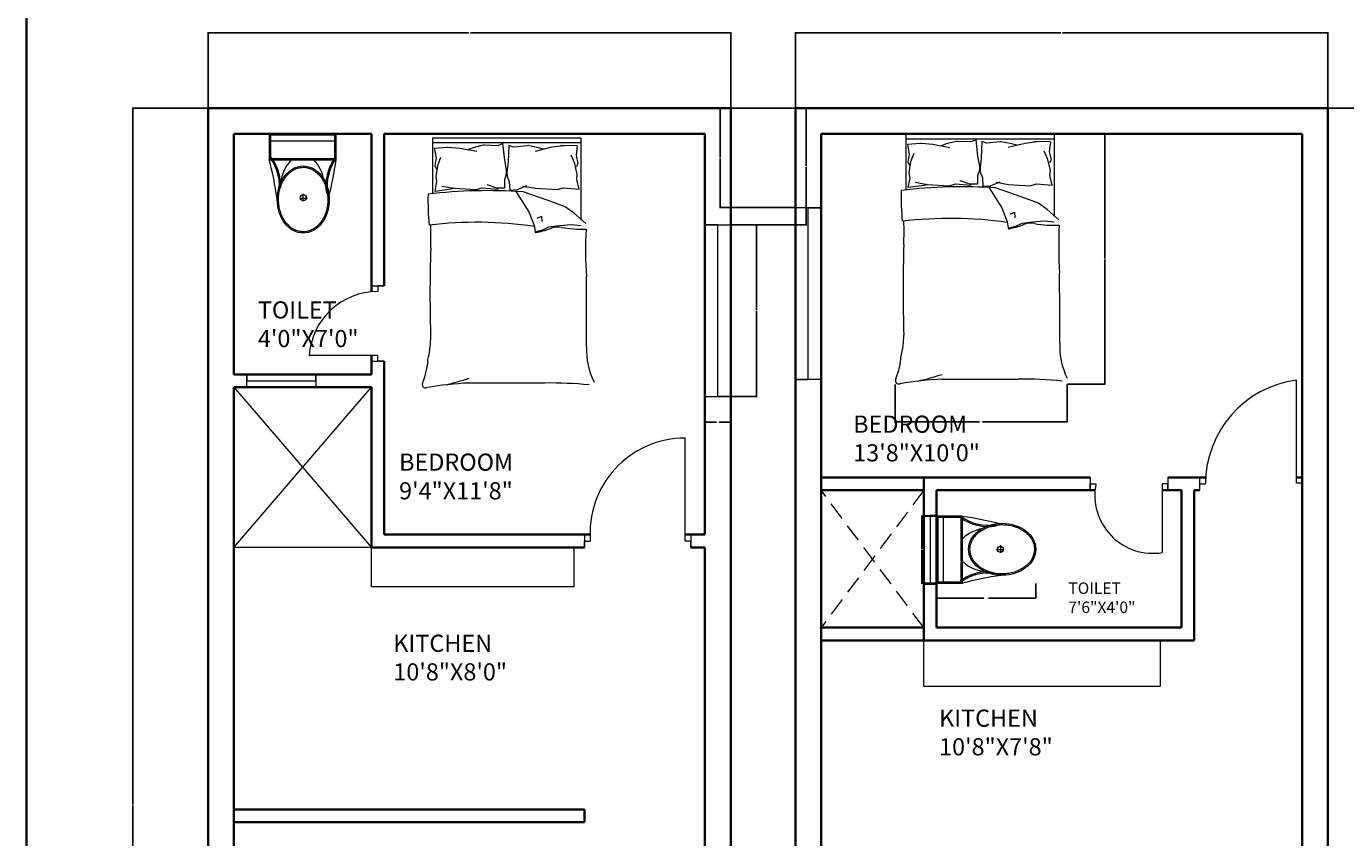
# Model space of a CAD drawing. Units: inches. Extents: x 2169 to 3181, y 1824 to 2912.
# Tile 2 of 5: x 2169 to 2630, y 2163 to 2446. Entities that reach past the tile are written whole.
import ezdxf

# ---------------------------------------------------------------- set-up
doc = ezdxf.new("R2010")
doc.units = ezdxf.units.IN
doc.linetypes.add('DASHED2', pattern=[9.525, 6.35, -3.175])
for name, color, linetype, lineweight in [('A-ANNO-DIMS', 2, 'Continuous', 18), ('A-ANNO-TTLB', 7, 'Continuous', 35), ('A-AREA-IDEN', 7, 'Continuous', 18), ('A-DOOR', 3, 'Continuous', 18), ('A-FLOR-CASE', 8, 'Continuous', 18), ('A-FLOR-FIXT', 9, 'Continuous', 18), ('A-FLOR-OPEN', 7, 'Continuous', 18), ('A-FLOR-OPEN-OVHD', 253, 'DASHED2', 13), ('A-FURN', 8, 'Continuous', 18), ('A-GLAZ', 4, 'Continuous', 18), ('A-WALL', 7, 'Continuous', 35)]:
    doc.layers.add(name, color=color, linetype=linetype, lineweight=lineweight)
doc.styles.get("Standard").update_dxf_attribs({"font": 'arial.ttf'})
doc.dimstyles.get("Standard").update_dxf_attribs({"dimtxt": 0.18, "dimasz": 0.18, "dimexe": 0.18, "dimexo": 0.0625, "dimgap": 0.09, "dimtad": 0, "dimtih": 1, "dimtoh": 1, "dimdec": 4, "dimzin": 0, "dimdsep": 46, "dimtxsty": 'Standard', "dimcen": 0.09, "dimadec": 0, "dimazin": 0, "dimtfac": 1, "dimtdec": 4, "dimtofl": 0, "dimtmove": 0, "dimatfit": 3, "dimfxl": 1, "dimtolj": 1, "dimtzin": 0, "dimarcsym": 0})

# ---------------------------------------------------------------- blocks, each defined once
blk = doc.blocks.new('A$C31115884')
for p, q in [((258, 466), (258, 523)), ((283, 498), (223, 498)), ((0, 200), (0, 0)), ((520, 200), (0, 200)), ((10, 190), (10, 10)), ((510, 190), (10, 190)), ((510, 10), (510, 190)), ((520, 0), (520, 200)), ((510, 54), (0, 54)), ((10, 10), (510, 10)), ((0, 0), (520, 0))]:
    blk.add_line(p, q)
blk.add_circle((256, 496), 23.6)
for centre, radius, start, end in [((2778, -205), 2807, 165.4549, 171.7133), ((-295, 403), 365, 324.2091, 9.3499), ((-295, 403), 375, 324.2091, 9.3499), ((139, 406), 293, 315.8436, 2.6563), ((806, 403), 365, 170.6501, 215.7909), ((3237, 905), 2807, 188.2867, 194.5451), ((384, 406), 293, 190.2774, 224.1564), ((806, 403), 375, 179.2036, 215.7909)]:
    blk.add_arc(centre, radius, start, end)
blk.add_ellipse((256, 510), major_axis=(0, -261), ratio=0.772727)
blk.add_open_spline([(256, 259), (263, 259), (270, 260), (288, 262), (299, 265), (320, 273), (330, 278), (350, 291), (360, 299), (378, 316), (386, 326), (402, 347), (409, 358), (421, 383), (427, 395), (436, 422), (440, 436), (445, 465), (447, 480), (448, 509), (448, 524), (445, 553), (443, 568), (436, 596), (432, 610), (422, 636), (416, 649), (402, 672), (395, 683), (379, 703), (370, 712), (351, 728), (341, 735), (321, 746), (310, 751), (289, 757), (278, 759), (256, 761), (245, 761), (223, 757), (212, 754), (191, 746), (181, 741), (161, 728), (151, 720), (133, 703), (125, 693), (110, 672), (103, 660), (90, 636), (85, 623), (76, 596), (72, 582), (67, 553), (66, 538), (64, 509), (65, 494), (68, 465), (70, 450), (77, 422), (81, 408), (91, 382), (97, 370), (111, 346), (118, 335), (135, 316), (144, 307), (162, 291), (172, 284), (193, 273), (203, 269), (225, 262), (236, 260), (250, 259), (253, 259), (256, 259)], degree=3, knots=[0, 0, 0, 0, 0.110105, 0.110105, 0.285049, 0.285049, 0.459994, 0.459994, 0.634938, 0.634938, 0.809882, 0.809882, 0.984827, 0.984827, 1.159771, 1.159771, 1.334715, 1.334715, 1.50966, 1.50966, 1.684604, 1.684604, 1.859549, 1.859549, 2.034493, 2.034493, 2.209437, 2.209437, 2.384382, 2.384382, 2.559326, 2.559326, 2.73427, 2.73427, 2.909215, 2.909215, 3.084159, 3.084159, 3.259103, 3.259103, 3.434048, 3.434048, 3.608992, 3.608992, 3.783936, 3.783936, 3.958881, 3.958881, 4.133825, 4.133825, 4.30877, 4.30877, 4.483714, 4.483714, 4.658658, 4.658658, 4.833603, 4.833603, 5.008547, 5.008547, 5.183491, 5.183491, 5.358436, 5.358436, 5.53338, 5.53338, 5.708324, 5.708324, 5.883269, 5.883269, 6.058213, 6.058213, 6.233158, 6.233158, 6.283185, 6.283185, 6.283185, 6.283185])
blk = doc.blocks.new('DOOR-BED-G-36IN')
for p, q in [((0, 0), (0, 36)), ((-35.15, 2.25), (-35.15, -2.25)), ((2, 2.25), (2, -2.25)), ((-35.15, -2.25), (-35.15, 0)), ((-35.15, 0), (-33.15, 0)), ((2, 0), (0, 0)), ((2, -2.25), (2, 0))]:
    blk.add_line(p, q)
blk.add_arc((0, 2.74), 33.26, 90, 184.7229)
blk = doc.blocks.new('DOOR-BATH-G-24IN')
for p, q in [((-2.25, 24.37), (2.25, 24.37)), ((2.25, 24.37), (0, 24.37)), ((0, 24.37), (0, 22.37)), ((0, 0), (-24, 0)), ((0, -2), (0, 0)), ((-2.25, -2), (-2.25, -2)), ((-2.25, -2), (2.25, -2)), ((2.25, -2), (0, -2))]:
    blk.add_line(p, q)
blk.add_arc((0, -1.69), 24.06, 90, 175.9745)
blk = doc.blocks.new('DOOR-BATH-U-24IN')
for p, q in [((-25.15, 2.25), (-25.15, -2.25)), ((2, 2.25), (2, -2.25)), ((-25.15, -2.25), (-25.15, 0)), ((-25.15, 0), (-23.15, 0)), ((2, 0), (0, 0)), ((0, 0), (0, -24)), ((2, -2.25), (2, 0))]:
    blk.add_line(p, q)
blk.add_arc((-3.27, -3.99), 20.28, 168.6528, 279.2746)
blk = doc.blocks.new('DOOR-BED-U-36IN')
for p, q in [((0, 0), (0, 36)), ((-33.79, -2.49), (-33.79, 2.01)), ((-33.79, 2.01), (-33.79, 2.01)), ((2, 0), (0, 0)), ((-33.79, -0.24), (-31.79, -0.24)), ((-33.79, -2.49), (-33.79, -2.49))]:
    blk.add_line(p, q)
blk.add_arc((4.76, -0.24), 36.56, 97.4851, 180)
blk = doc.blocks.new('WIN-60IN')
for p, q in [((4.5, 60), (0, 60)), ((0, 60), (9, 60)), ((4.5, 0), (4.5, 60)), ((0, 0), (9, 0)), ((9, 0), (4.5, 0)), ((9, 0), (9, 0))]:
    blk.add_line(p, q)
blk = doc.blocks.new('VENT-24IN-G')
for p, q in [((0, 0), (0, 4.5)), ((0, 4.5), (0, 2.25)), ((0, 2.25), (24, 2.25)), ((24, 2.25), (24, 4.5)), ((24, 4.5), (24, 0))]:
    blk.add_line(p, q)
blk = doc.blocks.new('VENT-24IN-U')
for p, q in [((0, 24), (0, 24)), ((0, 24), (4.5, 24)), ((4.5, 24), (2.25, 24)), ((2.25, 24), (2.25, 0)), ((2.25, 0), (0, 0)), ((0, 0), (4.5, 0))]:
    blk.add_line(p, q)
blk = doc.blocks.new('BED-DOUBLE')
for p, q in [((3.76, 67.77), (3.76, 87.35)), ((3.76, 87.35), (55.42, 87.35)), ((3.76, 85.69), (55.42, 85.69)), ((4.21, 83.74), (8.84, 84.1)), ((4.21, 83.77), (4.83, 80.33)), ((8.84, 84.1), (8.96, 84.08)), ((8.96, 84.08), (13.09, 83.77)), ((13.09, 83.77), (19.03, 82.67)), ((16.06, 83.3), (18.25, 84.08)), ((18.25, 84.08), (21.37, 84.86)), ((21.37, 84.86), (21.72, 84.86)), ((21.72, 84.86), (26.52, 84.7)), ((26.52, 84.7), (28.09, 85.33)), ((28.09, 85.33), (28.71, 79.55)), ((30.24, 84.66), (29.98, 78.85)), ((31.84, 84.13), (30.24, 84.66)), ((36.63, 84.59), (31.84, 84.13)), ((36.98, 84.61), (36.63, 84.59)), ((40.14, 84.02), (36.98, 84.61)), ((45.31, 84.03), (39.45, 82.57)), ((42.38, 83.38), (40.14, 84.02)), ((49.42, 84.6), (45.31, 84.03)), ((54.17, 84.59), (48.33, 84.69)), ((48.33, 84.69), (49.42, 84.6)), ((54.17, 84.59), (53.76, 81.12)), ((55.42, 87.35), (55.42, 58.59)), ((4.83, 80.33), (4.37, 77.51)), ((5.46, 77.67), (6.55, 80.64)), ((28.71, 79.55), (29.34, 76.11)), ((29.98, 78.85), (29.57, 75.38)), ((53.3, 78.42), (52.03, 81.32)), ((54.17, 74.56), (53.3, 78.42)), ((53.76, 81.12), (54.41, 78.34)), ((54.41, 78.34), (53.85, 77.21)), ((4.37, 77.51), (4.99, 76.42)), ((4.83, 73.76), (5.46, 77.67)), ((5.15, 72.04), (4.83, 73.76)), ((29.34, 74.7), (28.71, 72.67)), ((29.34, 76.11), (29.34, 74.7)), ((29.57, 75.38), (29.66, 73.97)), ((29.66, 73.97), (30.41, 71.98)), ((53.97, 72.83), (54.17, 74.56)), ((4.52, 68.6), (5.15, 72.04)), ((10.03, 69.39), (4.52, 68.6)), ((6.9, 70.46), (11.26, 69.74)), ((11.26, 69.74), (10.03, 69.39)), ((11.26, 69.74), (18.83, 69.27)), ((18.83, 69.27), (20.95, 69.87)), ((20.95, 69.87), (26.5, 69.44)), ((26.06, 69.77), (22.66, 70.95)), ((28.71, 69.77), (26.06, 69.77)), ((28.71, 72.67), (28.71, 69.77)), ((30.41, 71.98), (30.59, 69.09)), ((30.59, 69.09), (33.24, 69.26)), ((33.24, 69.26), (36.56, 70.64)), ((35.2, 70.46), (39.56, 69.74)), ((39.56, 69.74), (47.14, 69.27)), ((47.14, 69.27), (49.26, 69.87)), ((49.26, 69.87), (54.81, 69.44)), ((54.81, 69.44), (53.97, 72.83)), ((32.71, 68.56), (37.24, 61.54)), ((43.94, 65.39), (34.92, 68.56)), ((49.96, 63.21), (43.94, 65.39)), ((37.24, 61.54), (39.08, 56.69)), ((40.12, 59.32), (41.78, 59.99)), ((41.87, 58.1), (41.78, 59.99, 4.18)), ((53.15, 60.87), (49.96, 63.21)), ((57.15, 57.36), (53.15, 60.87)), ((39.08, 56.69), (39.42, 54.51)), ((42.1, 55.18), (44.27, 56.19)), ((44.27, 56.19), (47.96, 56.69)), ((47.96, 56.69), (52.14, 57.02)), ((52.14, 57.02), (55.49, 56.69)), ((39.42, 54.51), (42.1, 55.18)), ((16.28, 1.69), (42.89, 1.69))]:
    blk.add_line(p, q)
for centre, radius, start, end in [((92.06, 65.63), 90.06, 178.7218, 185.604), ((23.09, -109.45), 178.34, 86.0865, 96.7821), ((19.19, -81.63), 139.47, 81.7845, 96.9006), ((-180.86, 53.65), 183.89, 358.4762, 1.0082), ((33.68, 85.75), 32.06, 280.6617, 289.8806), ((47.29, 49.44), 6.73, 78.6608, 113.7384), ((55.49, 94.55), 39.11, 259.8763, 272.5657), ((197.03, 48.09), 139.99, 176.9791, 183.8365), ((39.6, 54.45), 0.199, 160.2464, 271.1377), ((524.1, 32.64), 521.39, 178.2277, 181.7185), ((-4874.07, 14.03), 4931.49, 0.00217, 0.28689), ((-29.08, 17.61), 32.04, 346.0648, 358.9113), ((82.33, 13.12), 24.93, 177.4714, 206.4681), ((-23.41, 11.38), 25.47, 337.9751, 356.652), ((1.18, 1.17), 1.18, 146.1736, 293.4781), ((23.16, -129.76), 131.62, 92.9958, 99.4091), ((-18.62, 112.98), 115.08, 283.3832, 287.7053), ((44.49, -142.13), 143.82, 84.4998, 90.6351)]:
    blk.add_arc(centre, radius, start, end)
blk = doc.blocks.new('*D19')
at = {"layer": 'A-ANNO-DIMS', "color": 0, "lineweight": -2, "transparency": 16777216}
for p, q in [((2414.84, 2376.69), (2423.95, 2376.69)), ((2423.77, 2376.51), (2423.77, 2346.87)), ((2423.77, 2316.87), (2423.77, 2346.51)), ((2414.84, 2316.69), (2423.95, 2316.69))]:
    blk.add_line(p, q, dxfattribs=at)
at = {"layer": 'A-ANNO-DIMS', "color": 0, "transparency": 16777216}
for points in [[(2423.74, 2376.51), (2423.8, 2376.51), (2423.77, 2376.69)], [(2423.74, 2316.87), (2423.8, 2316.87), (2423.77, 2316.69)]]:
    blk.add_solid(points, dxfattribs=at)
at = {"layer": 'Defpoints', "color": 0, "transparency": 16777216}
for p in [(2414.77, 2376.69), (2423.77, 2376.69), (2414.77, 2316.69)]:
    blk.add_point(p, dxfattribs=at)
at = {"layer": 'A-ANNO-DIMS', "color": 0, "transparency": 16777216, "insert": (2423.77, 2346.69), "char_height": 0.18, "attachment_point": 5}
blk.add_mtext('\\A1;WINDOW 60 TYP.', dxfattribs=at)
blk = doc.blocks.new('*D20')
at = {"layer": 'A-ANNO-DIMS', "color": 0, "lineweight": -2, "transparency": 16777216}
for p, q in [((2405.77, 2316.63), (2405.77, 2307.51)), ((2414.77, 2316.63), (2414.77, 2307.51)), ((2405.95, 2307.69), (2409.82, 2307.69)), ((2414.59, 2307.69), (2410.73, 2307.69))]:
    blk.add_line(p, q, dxfattribs=at)
at = {"layer": 'A-ANNO-DIMS', "color": 0, "transparency": 16777216}
for points in [[(2405.95, 2307.72), (2405.95, 2307.66), (2405.77, 2307.69)], [(2414.59, 2307.72), (2414.59, 2307.66), (2414.77, 2307.69)]]:
    blk.add_solid(points, dxfattribs=at)
at = {"layer": 'Defpoints', "color": 0, "transparency": 16777216}
for p in [(2405.77, 2316.69), (2414.77, 2316.69), (2414.77, 2307.69)]:
    blk.add_point(p, dxfattribs=at)
at = {"layer": 'A-ANNO-DIMS', "color": 0, "transparency": 16777216, "insert": (2410.27, 2307.69), "char_height": 0.18, "attachment_point": 5}
blk.add_mtext('\\A1;9 TYP.', dxfattribs=at)
blk = doc.blocks.new('*D43')
at = {"layer": 'A-ANNO-DIMS', "color": 0, "lineweight": -2, "transparency": 16777216}
for p, q in [((2486.67, 2251.35), (2486.67, 2246.04)), ((2521.31, 2251.35), (2521.31, 2246.04)), ((2486.85, 2246.22), (2503.21, 2246.22)), ((2521.13, 2246.22), (2504.77, 2246.22))]:
    blk.add_line(p, q, dxfattribs=at)
at = {"layer": 'A-ANNO-DIMS', "color": 0, "transparency": 16777216}
for points in [[(2486.85, 2246.25), (2486.85, 2246.19), (2486.67, 2246.22)], [(2521.13, 2246.25), (2521.13, 2246.19), (2521.31, 2246.22)]]:
    blk.add_solid(points, dxfattribs=at)
at = {"layer": 'Defpoints', "color": 0, "transparency": 16777216}
for p in [(2486.67, 2251.42), (2521.31, 2251.42), (2521.31, 2246.22)]:
    blk.add_point(p, dxfattribs=at)
at = {"layer": 'A-ANNO-DIMS', "color": 0, "transparency": 16777216, "insert": (2503.99, 2246.22), "char_height": 0.18, "attachment_point": 5}
blk.add_mtext('\\A1;WC 35 TYP.', dxfattribs=at)
blk = doc.blocks.new('*D44')
at = {"layer": 'A-ANNO-DIMS', "color": 0, "lineweight": -2, "transparency": 16777216}
for p, q in [((2486.61, 2274.79), (2481.29, 2274.79)), ((2481.47, 2274.61), (2481.47, 2263.29)), ((2481.47, 2251.6), (2481.47, 2262.92)), ((2486.61, 2251.42), (2481.29, 2251.42))]:
    blk.add_line(p, q, dxfattribs=at)
at = {"layer": 'A-ANNO-DIMS', "color": 0, "transparency": 16777216}
for points in [[(2481.44, 2274.61), (2481.5, 2274.61), (2481.47, 2274.79)], [(2481.44, 2251.6), (2481.5, 2251.6), (2481.47, 2251.42)]]:
    blk.add_solid(points, dxfattribs=at)
at = {"layer": 'Defpoints', "color": 0, "transparency": 16777216}
for p in [(2486.67, 2274.79), (2481.47, 2251.42), (2486.67, 2251.42)]:
    blk.add_point(p, dxfattribs=at)
at = {"layer": 'A-ANNO-DIMS', "color": 0, "transparency": 16777216, "insert": (2481.47, 2263.11), "char_height": 0.18, "attachment_point": 5}
blk.add_mtext('\\A1;23 TYP.', dxfattribs=at)
blk = doc.blocks.new('*D45')
at = {"layer": 'A-ANNO-DIMS', "color": 0, "lineweight": -2, "transparency": 16777216}
for p, q in [((2532.34, 2408.39), (2545.57, 2408.39)), ((2545.39, 2408.21), (2545.39, 2364.84)), ((2545.39, 2321.11), (2545.39, 2364.48)), ((2532.34, 2320.93), (2545.57, 2320.93))]:
    blk.add_line(p, q, dxfattribs=at)
at = {"layer": 'A-ANNO-DIMS', "color": 0, "transparency": 16777216}
for points in [[(2545.36, 2408.21), (2545.42, 2408.21), (2545.39, 2408.39)], [(2545.36, 2321.11), (2545.42, 2321.11), (2545.39, 2320.93)]]:
    blk.add_solid(points, dxfattribs=at)
at = {"layer": 'Defpoints', "color": 0, "transparency": 16777216}
for p in [(2532.27, 2408.39), (2545.39, 2408.39), (2532.27, 2320.93)]:
    blk.add_point(p, dxfattribs=at)
at = {"layer": 'A-ANNO-DIMS', "color": 0, "transparency": 16777216, "insert": (2545.39, 2364.66), "char_height": 0.18, "attachment_point": 5}
blk.add_mtext('\\A1;BED 87 TYP.', dxfattribs=at)
blk = doc.blocks.new('*D46')
at = {"layer": 'A-ANNO-DIMS', "color": 0, "lineweight": -2, "transparency": 16777216}
for p, q in [((2472.17, 2320.86), (2472.17, 2307.63)), ((2532.27, 2320.86), (2532.27, 2307.63)), ((2472.35, 2307.81), (2501.69, 2307.81)), ((2532.09, 2307.81), (2502.75, 2307.81))]:
    blk.add_line(p, q, dxfattribs=at)
at = {"layer": 'A-ANNO-DIMS', "color": 0, "transparency": 16777216}
for points in [[(2472.35, 2307.84), (2472.35, 2307.78), (2472.17, 2307.81)], [(2532.09, 2307.84), (2532.09, 2307.78), (2532.27, 2307.81)]]:
    blk.add_solid(points, dxfattribs=at)
at = {"layer": 'Defpoints', "color": 0, "transparency": 16777216}
for p in [(2472.17, 2320.93), (2532.27, 2320.93), (2532.27, 2307.81)]:
    blk.add_point(p, dxfattribs=at)
at = {"layer": 'A-ANNO-DIMS', "color": 0, "transparency": 16777216, "insert": (2502.22, 2307.81), "char_height": 0.18, "attachment_point": 5}
blk.add_mtext('\\A1;60 TYP.', dxfattribs=at)
blk = doc.blocks.new('*D53')
at = {"layer": 'A-ANNO-DIMS', "color": 0, "lineweight": -2, "transparency": 16777216}
for p, q in [((2232.27, 2417.45), (2232.27, 2443.92)), ((2232.45, 2443.74), (2323.14, 2443.74)), ((2414.59, 2443.74), (2323.91, 2443.74)), ((2414.77, 2417.45), (2414.77, 2443.92))]:
    blk.add_line(p, q, dxfattribs=at)
at = {"layer": 'A-ANNO-DIMS', "color": 0, "transparency": 16777216}
for points in [[(2232.45, 2443.77), (2232.45, 2443.71), (2232.27, 2443.74)], [(2414.59, 2443.77), (2414.59, 2443.71), (2414.77, 2443.74)]]:
    blk.add_solid(points, dxfattribs=at)
at = {"layer": 'Defpoints', "color": 0, "transparency": 16777216}
for p in [(2414.77, 2443.74), (2232.27, 2417.39), (2414.77, 2417.39)]:
    blk.add_point(p, dxfattribs=at)
at = {"layer": 'A-ANNO-DIMS', "color": 0, "transparency": 16777216, "insert": (2323.52, 2443.74), "char_height": 0.18, "attachment_point": 5}
blk.add_mtext('\\A1;182.5', dxfattribs=at)
blk = doc.blocks.new('*D54')
at = {"layer": 'A-ANNO-DIMS', "color": 0, "lineweight": -2, "transparency": 16777216}
for p, q in [((2232.21, 2417.39), (2205.74, 2417.39)), ((2205.92, 2417.21), (2205.92, 2174.07)), ((2205.92, 1930.57), (2205.92, 2173.71)), ((2232.21, 1930.39), (2205.74, 1930.39))]:
    blk.add_line(p, q, dxfattribs=at)
at = {"layer": 'A-ANNO-DIMS', "color": 0, "transparency": 16777216}
for points in [[(2205.89, 2417.21), (2205.95, 2417.21), (2205.92, 2417.39)], [(2205.89, 1930.57), (2205.95, 1930.57), (2205.92, 1930.39)]]:
    blk.add_solid(points, dxfattribs=at)
at = {"layer": 'Defpoints', "color": 0, "transparency": 16777216}
for p in [(2205.92, 2417.39), (2232.27, 2417.39), (2232.27, 1930.39)]:
    blk.add_point(p, dxfattribs=at)
at = {"layer": 'A-ANNO-DIMS', "color": 0, "transparency": 16777216, "insert": (2205.92, 2173.89), "char_height": 0.18, "attachment_point": 5}
blk.add_mtext('\\A1;487', dxfattribs=at)
blk = doc.blocks.new('*D55')
at = {"layer": 'A-ANNO-DIMS', "color": 0, "lineweight": -2, "transparency": 16777216}
for p, q in [((2437.37, 2417.45), (2437.37, 2443.92)), ((2437.55, 2443.74), (2530.09, 2443.74)), ((2623.19, 2443.74), (2530.65, 2443.74)), ((2623.37, 2417.45), (2623.37, 2443.92))]:
    blk.add_line(p, q, dxfattribs=at)
at = {"layer": 'A-ANNO-DIMS', "color": 0, "transparency": 16777216}
for points in [[(2437.55, 2443.77), (2437.55, 2443.71), (2437.37, 2443.74)], [(2623.19, 2443.77), (2623.19, 2443.71), (2623.37, 2443.74)]]:
    blk.add_solid(points, dxfattribs=at)
at = {"layer": 'Defpoints', "color": 0, "transparency": 16777216}
for p in [(2623.37, 2443.74), (2437.37, 2417.39), (2623.37, 2417.39)]:
    blk.add_point(p, dxfattribs=at)
at = {"layer": 'A-ANNO-DIMS', "color": 0, "transparency": 16777216, "insert": (2530.37, 2443.74), "char_height": 0.18, "attachment_point": 5}
blk.add_mtext('\\A1;186', dxfattribs=at)
blk = doc.blocks.new('*D56')
at = {"layer": 'A-ANNO-DIMS', "color": 0, "lineweight": -2, "transparency": 16777216}
for p, q in [((2623.43, 2417.39), (2649.9, 2417.39)), ((2649.72, 2417.21), (2649.72, 2174.07)), ((2649.72, 1930.57), (2649.72, 2173.71)), ((2623.43, 1930.39), (2649.9, 1930.39))]:
    blk.add_line(p, q, dxfattribs=at)
at = {"layer": 'A-ANNO-DIMS', "color": 0, "transparency": 16777216}
for points in [[(2649.69, 2417.21), (2649.75, 2417.21), (2649.72, 2417.39)], [(2649.69, 1930.57), (2649.75, 1930.57), (2649.72, 1930.39)]]:
    blk.add_solid(points, dxfattribs=at)
at = {"layer": 'Defpoints', "color": 0, "transparency": 16777216}
for p in [(2623.37, 2417.39), (2649.72, 2417.39), (2623.37, 1930.39)]:
    blk.add_point(p, dxfattribs=at)
at = {"layer": 'A-ANNO-DIMS', "color": 0, "transparency": 16777216, "insert": (2649.72, 2173.89), "char_height": 0.18, "attachment_point": 5}
blk.add_mtext('\\A1;487', dxfattribs=at)
blk = doc.blocks.new('*D57')
at = {"layer": 'A-ANNO-DIMS', "color": 0, "lineweight": -2, "transparency": 16777216}
for p, q in [((2414.84, 2417.39), (2441.3, 2417.39)), ((2441.12, 2417.21), (2441.12, 2397.22)), ((2441.12, 2376.87), (2441.12, 2396.86)), ((2414.84, 2376.69), (2441.3, 2376.69))]:
    blk.add_line(p, q, dxfattribs=at)
at = {"layer": 'A-ANNO-DIMS', "color": 0, "transparency": 16777216}
for points in [[(2441.09, 2417.21), (2441.15, 2417.21), (2441.12, 2417.39)], [(2441.09, 2376.87), (2441.15, 2376.87), (2441.12, 2376.69)]]:
    blk.add_solid(points, dxfattribs=at)
at = {"layer": 'Defpoints', "color": 0, "transparency": 16777216}
for p in [(2414.77, 2417.39), (2414.77, 2376.69), (2441.12, 2376.69)]:
    blk.add_point(p, dxfattribs=at)
at = {"layer": 'A-ANNO-DIMS', "color": 0, "transparency": 16777216, "insert": (2441.12, 2397.04), "char_height": 0.18, "attachment_point": 5}
blk.add_mtext('\\A1;40.7', dxfattribs=at)
blk = doc.blocks.new('*D58')
at = {"layer": 'A-ANNO-DIMS', "color": 0, "lineweight": -2, "transparency": 16777216}
for p, q in [((2437.31, 2417.39), (2410.84, 2417.39)), ((2411.02, 2417.21), (2411.02, 2400.2)), ((2411.02, 2382.82), (2411.02, 2399.83)), ((2437.31, 2382.64), (2410.84, 2382.64))]:
    blk.add_line(p, q, dxfattribs=at)
at = {"layer": 'A-ANNO-DIMS', "color": 0, "transparency": 16777216}
for points in [[(2410.99, 2417.21), (2411.05, 2417.21), (2411.02, 2417.39)], [(2410.99, 2382.82), (2411.05, 2382.82), (2411.02, 2382.64)]]:
    blk.add_solid(points, dxfattribs=at)
at = {"layer": 'Defpoints', "color": 0, "transparency": 16777216}
for p in [(2437.37, 2417.39), (2411.02, 2382.64), (2437.37, 2382.64)]:
    blk.add_point(p, dxfattribs=at)
at = {"layer": 'A-ANNO-DIMS', "color": 0, "transparency": 16777216, "insert": (2411.02, 2400.01), "char_height": 0.18, "attachment_point": 5}
blk.add_mtext('\\A1;34.76', dxfattribs=at)

msp = doc.modelspace()

# ---------------------------------------------------------------- linework, layer by layer
at = {"layer": 'A-ANNO-TTLB'}
msp.add_lwpolyline([(2168.7598, 2912.462), (3180.8253, 2912.462), (3180.8253, 1823.5481), (2168.7598, 1823.5481)], close=True, dxfattribs=at)
at = {"layer": 'A-FLOR-CASE'}
for points in [[(2289.2736, 2263.8924), (2359.9816, 2263.8924), (2359.9816, 2250.1381), (2289.2736, 2250.1381)], [(2482.1687, 2231.3924), (2564.7627, 2231.3924), (2564.7627, 2215.3735), (2482.1687, 2215.3735)]]:
    msp.add_lwpolyline(points, close=True, dxfattribs=at)
at = {"layer": 'A-FLOR-OPEN'}
for p, q in [((2241.2736, 2263.8924), (2289.2736, 2319.8924)), ((2241.2736, 2319.8924), (2289.2736, 2263.8924)), ((2289.2736, 2263.8924), (2241.2736, 2263.8924))]:
    msp.add_line(p, q, dxfattribs=at)
at = {"layer": 'A-FLOR-OPEN-OVHD'}
for p, q in [((2482.1687, 2283.8924), (2446.3698, 2235.8924)), ((2482.1687, 2235.8924), (2446.3698, 2283.8924)), ((2482.1687, 2273.085), (2482.1687, 2273.085))]:
    msp.add_line(p, q, dxfattribs=at)
at = {"layer": 'A-WALL'}
for p, q in [((2232.2736, 2417.3924), (2414.7736, 2417.3924)), ((2232.2736, 2417.3924), (2414.7736, 2417.3924)), ((2232.2736, 2417.3924), (2232.2736, 1930.3924)), ((2414.7736, 2417.3924), (2414.7736, 1930.3924)), ((2437.3698, 2417.3924), (2623.3698, 2417.3924)), ((2437.3698, 2417.3924), (2437.3698, 1930.3924)), ((2614.3698, 2417.3924), (2623.3698, 2417.3924)), ((2623.3698, 2417.3924), (2623.3698, 1930.3924)), ((2241.2736, 2408.3924), (2289.2736, 2408.3924)), ((2241.2736, 2408.3924), (2241.2736, 2324.3924)), ((2289.2736, 2408.3924), (2289.2736, 2353.2673)), ((2293.7736, 2408.3924), (2293.7736, 2355.3727)), ((2293.7736, 2408.3924), (2405.7736, 2408.3924)), ((2405.7736, 2408.3924), (2405.7736, 2268.3924)), ((2446.3698, 2408.3924), (2614.3698, 2408.3924)), ((2446.3698, 2408.3924), (2446.3698, 2023.8924)), ((2446.3698, 2408.3924), (2610.3698, 2408.3924)), ((2446.3698, 2408.3924), (2614.3698, 2408.3924)), ((2614.3698, 2408.3924), (2614.3698, 1930.3924)), ((2289.2736, 2331.0023), (2289.2736, 2324.3924)), ((2293.7736, 2329.0023), (2293.7736, 2268.3924)), ((2241.2736, 2324.3924), (2289.2736, 2324.3924)), ((2241.2736, 2319.8924), (2289.2736, 2319.8924)), ((2241.2736, 2319.8924), (2241.2736, 2023.8924)), ((2289.2736, 2319.8924), (2289.2736, 2263.8924)), ((2482.1687, 2288.3924), (2446.3698, 2288.3924)), ((2446.3698, 2288.3924), (2446.3698, 2283.8924)), ((2482.1687, 2288.3924), (2540.3301, 2288.3924)), ((2482.1687, 2288.3924), (2482.1687, 2231.3924)), ((2482.1687, 2288.3924), (2540.3301, 2288.3924)), ((2567.4772, 2288.3924), (2572.1687, 2288.3924)), ((2567.4772, 2288.3924), (2580.6449, 2288.3924)), ((2612.3698, 2288.3924), (2614.3698, 2288.3924)), ((2446.3698, 2283.8924), (2482.1687, 2283.8924)), ((2446.3698, 2283.8924), (2450.8698, 2283.8924)), ((2482.1687, 2283.8924), (2482.1687, 2231.3924)), ((2486.6687, 2283.8924), (2486.6687, 2235.8924)), ((2486.6687, 2283.8924), (2542.0085, 2283.8924)), ((2565.4772, 2283.8924), (2572.1687, 2283.8924)), ((2572.1687, 2283.8924), (2572.1687, 2235.8924)), ((2576.6687, 2231.3924), (2576.6687, 2283.8924)), ((2576.6687, 2283.8924), (2578.5756, 2283.8924)), ((2293.7736, 2268.3924), (2365.6155, 2268.3924)), ((2398.8733, 2268.3924), (2405.7736, 2268.3924)), ((2289.2736, 2263.8924), (2363.7249, 2263.8924)), ((2400.8733, 2263.8924), (2405.7736, 2263.8924)), ((2405.7736, 2263.8924), (2405.7736, 1930.3924)), ((2446.3698, 2231.3924), (2446.3698, 2235.8924)), ((2446.3698, 2235.8924), (2482.1687, 2235.8924)), ((2482.1687, 2235.8924), (2482.1687, 2235.8924)), ((2486.6687, 2235.8924), (2572.1687, 2235.8924)), ((2482.1687, 2231.3924), (2446.3698, 2231.3924)), ((2482.1687, 2231.3924), (2576.6687, 2231.3924)), ((2572.1687, 2231.3924), (2576.6687, 2231.3924)), ((2241.2736, 2172.3924), (2363.7249, 2172.3924)), ((2363.7249, 2172.3924), (2363.7249, 2167.8924)), ((2241.2736, 2167.8924), (2363.7249, 2167.8924))]:
    msp.add_line(p, q, dxfattribs=at)

# ---------------------------------------------------------------- block references
at = {"layer": 'A-DOOR'}
for name, p in [('DOOR-BATH-G-24IN', (2291.5236, 2331.0023)), ('DOOR-BED-U-36IN', (2612.3698, 2286.3872)), ('DOOR-BED-G-36IN', (2398.8733, 2266.1424)), ('DOOR-BATH-U-24IN', (2565.4772, 2286.1424))]:
    msp.add_blockref(name, p, dxfattribs=at)
at = {"layer": 'A-FLOR-FIXT', "xscale": 0.0449564796810799, "yscale": 0.0449564796810799, "zscale": 0.0449564796810799}
for p, rotation in [((2276.9623, 2408.3924), 179.9999999999999), ((2486.6687, 2274.7941), 269.9999999999999)]:
    msp.add_blockref('A$C31115884', p, dxfattribs=dict(at, rotation=rotation))
at = {"layer": 'A-FURN'}
for p in [(2307.01, 2319.694), (2472.2658, 2321.0414)]:
    msp.add_blockref('BED-DOUBLE', p, dxfattribs=at)
at = {"layer": 'A-GLAZ', "extrusion": (0, 0, -1), "zscale": -1}
msp.add_blockref('WIN-60IN', (-2446.3694, 2322.6361), dxfattribs=at)
at = {"layer": 'A-GLAZ'}
for name, p in [('WIN-60IN', (2405.774, 2316.692)), ('VENT-24IN-G', (2245.809, 2319.892)), ('VENT-24IN-U', (2482.169, 2251.127))]:
    msp.add_blockref(name, p, dxfattribs=at)

# ---------------------------------------------------------------- texts
at = {"layer": 'A-AREA-IDEN', "attachment_point": 1}
for s, width, insert, char_height in [('TOILET\\P4\'0"X7\'0"', 98.915771, (2249.6076, 2349.9021), 6), ('BEDROOM\\P13\'8"X10\'0"', 126.46563, (2457.5344, 2309.9891), 6), ('BEDROOM\\P9\'4"X11\'8"', 103.537439, (2298.933, 2296.7227), 6), ('TOILET\\P7\'6"X4\'0"', 90.687067, (2532.6827, 2251.6822), 4), ('KITCHEN\\P10\'8"X8\'0"', 89.096746, (2296.9131, 2233.4352), 6), ('KITCHEN\\P10\'8"X7\'8"', 154.928298, (2487.5311, 2207.2786), 6)]:
    msp.add_mtext_dynamic_manual_height_columns(s, width=width, gutter_width=12.5, heights=[0], dxfattribs=dict(at, insert=insert, char_height=char_height))

# ---------------------------------------------------------------- dimensions: what is measured, and where the dimension line sits
at = {"layer": 'A-ANNO-DIMS'}
for base, p1, p2, override, picture, middle in [((2414.7736, 2443.7424), (2232.2736, 2417.3924), (2414.7736, 2417.3924), {"dimdec": 1, "dimlfac": 1, "dimrnd": 0, "dimzin": 0, "dimdsep": 46, "dimlunit": 2}, '*D53', (2323.5236, 2443.7424)), ((2623.3698, 2443.7424), (2437.3698, 2417.3924), (2623.3698, 2417.3924), {"dimdec": 0, "dimlfac": 1, "dimrnd": 0, "dimzin": 0, "dimdsep": 46, "dimlunit": 2}, '*D55', (2530.3698, 2443.7424))]:
    dim = msp.add_linear_dim(base=base, p1=p1, p2=p2, dimstyle='Standard', override=override, dxfattribs=at)
    dim.commit()
    dim.dimension.update_dxf_attribs({"geometry": picture, "text_midpoint": middle})
for base, p1, p2, override, picture, middle in [((2205.9236, 2417.3924), (2232.2736, 1930.3924), (2232.2736, 2417.3924), {"dimdec": 0, "dimlfac": 1, "dimrnd": 0, "dimzin": 0, "dimdsep": 46, "dimlunit": 2}, '*D54', (2205.9236, 2173.8924)), ((2411.0198, 2382.6356), (2437.3698, 2417.3924), (2437.3698, 2382.6356), {"dimdec": 2, "dimlfac": 1, "dimrnd": 0, "dimzin": 0, "dimdsep": 46, "dimlunit": 2}, '*D58', (2411.0198, 2400.014)), ((2441.1236, 2376.6915), (2414.7736, 2417.3924), (2414.7736, 2376.6915), {"dimdec": 1, "dimlfac": 1, "dimrnd": 0, "dimzin": 0, "dimdsep": 46, "dimlunit": 2}, '*D57', (2441.1236, 2397.042)), ((2649.7198, 2417.3924), (2623.3698, 1930.3924), (2623.3698, 2417.3924), {"dimdec": 0, "dimlfac": 1, "dimrnd": 0, "dimzin": 0, "dimdsep": 46, "dimlunit": 2}, '*D56', (2649.7198, 2173.8924))]:
    dim = msp.add_linear_dim(base=base, p1=p1, p2=p2, angle=90, dimstyle='Standard', override=override, dxfattribs=at)
    dim.commit()
    dim.dimension.update_dxf_attribs({"geometry": picture, "text_midpoint": middle})
for base, p1, p2, angle, text, picture, middle in [((2545.3924, 2408.3924), (2532.2726, 2320.9274), (2532.2726, 2408.3924), 90, 'BED <> TYP.', '*D45', (2545.3924, 2364.6599)), ((2423.7736, 2376.6915), (2414.7736, 2316.6915), (2414.7736, 2376.6915), 90, 'WINDOW <> TYP.', '*D19', (2423.7736, 2346.6915)), ((2481.4724, 2251.4167), (2486.6687, 2274.7941), (2486.6687, 2251.4167), 270, '<> TYP.', '*D44', (2481.4724, 2263.1054))]:
    dim = msp.add_linear_dim(base=base, p1=p1, p2=p2, angle=angle, text=text, dimstyle='Standard', override={"dimdec": 0, "dimlfac": 1, "dimrnd": 0, "dimzin": 0, "dimdsep": 46, "dimlunit": 2}, dxfattribs=at)
    dim.commit()
    dim.dimension.update_dxf_attribs({"geometry": picture, "text_midpoint": middle})
for base, p1, p2, text, picture, middle in [((2532.2726, 2307.8076), (2472.1721, 2320.9274), (2532.2726, 2320.9274), '<> TYP.', '*D46', (2502.2224, 2307.8076)), ((2414.7736, 2307.6915), (2405.7736, 2316.6915), (2414.7736, 2316.6915), '<> TYP.', '*D20', (2410.2736, 2307.6915)), ((2521.3108, 2246.2204), (2486.6687, 2251.4167), (2521.3108, 2251.4167), 'WC <> TYP.', '*D43', (2503.9897, 2246.2204))]:
    dim = msp.add_linear_dim(base=base, p1=p1, p2=p2, text=text, dimstyle='Standard', override={"dimdec": 0, "dimlfac": 1, "dimrnd": 0, "dimzin": 0, "dimdsep": 46, "dimlunit": 2}, dxfattribs=at)
    dim.commit()
    dim.dimension.update_dxf_attribs({"geometry": picture, "text_midpoint": middle})

doc.saveas('drawing.dxf')
